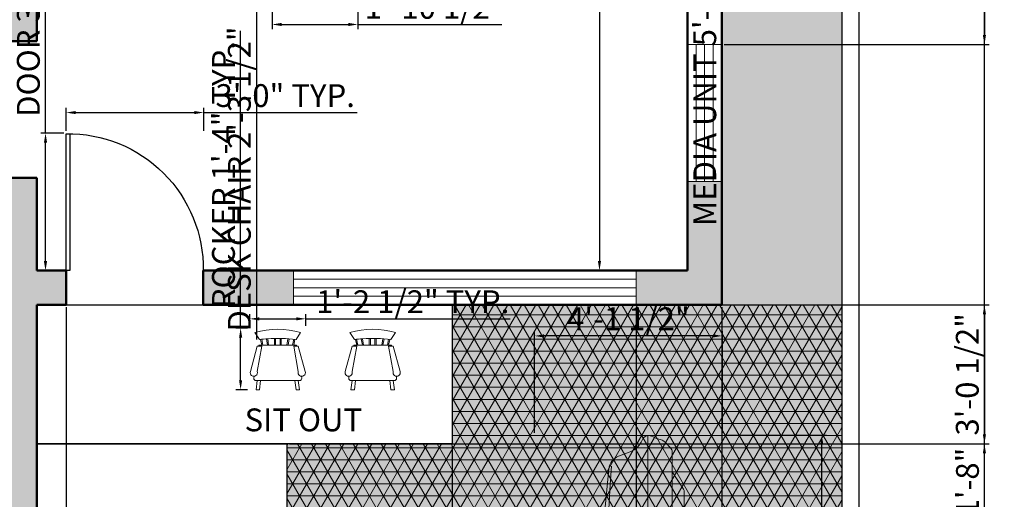
# Model space of a CAD drawing. Units: inches. Extents: x 2623 to 3157, y 1514 to 2273.
# Tile 3 of 6: x 2898 to 3157, y 1729 to 1856. Entities that reach past the tile are written whole.
import ezdxf

# ---------------------------------------------------------------- set-up
doc = ezdxf.new("R2010")
doc.units = ezdxf.units.IN
for name, color, linetype, lineweight in [('A-ANNO-DIMS', 2, 'Continuous', 18), ('A-AREA-IDEN', 7, 'Continuous', 25), ('A-DOOR', 4, 'Continuous', 25), ('A-FLOR', 7, 'Continuous', 25), ('A-FURN', 8, 'Continuous', 18), ('A-GLAZ', 4, 'Continuous', 20), ('A-WALL', 7, 'Continuous', 50), ('A-WALL-PATT', 252, 'Continuous', 13), ('C-PRKG', 8, 'Continuous', 20), ('C-PRKG-BASE-PATT', 51, 'Continuous', 13), ('C-PRKG-PATT', 252, 'Continuous', 13), ('C-PRKG-VEHL', 9, 'Continuous', 13), ('C-PROP', 7, 'Continuous', 25), ('L-PLNT-PATT', 9, 'Continuous', 13)]:
    doc.layers.add(name, color=color, linetype=linetype, lineweight=lineweight)
doc.styles.get("Standard").update_dxf_attribs({"font": 'arial.ttf'})
doc.dimstyles.new('ISO-25', dxfattribs={"dimtxt": 6, "dimasz": 2.5, "dimexe": 1.25, "dimexo": 0.625, "dimtad": 1, "dimdec": 1, "dimlunit": 3, "dimtxsty": 'Standard', "dimcen": 2.5, "dimadec": 0, "dimazin": 0, "dimtfac": 1, "dimtdec": 1, "dimtmove": 0, "dimatfit": 3, "dimfxl": 1, "dimarcsym": 0})

# ---------------------------------------------------------------- blocks, each defined once
blk = doc.blocks.new('Chair - Rocking')
for p, q in [((-8, -4.5), (-10, -1.5)), ((-4.5, -7), (-4.96674, -4.19951)), ((-4, -7), (-4.40532, -4.16272)), ((-1.5, -4.05012), (-1.5, -7)), ((-1, -7), (-1, -4.05012)), ((1, -7), (1, -4.04655)), ((1.5, -4.05012), (1.5, -7)), ((4, -7), (4.40187, -4.18694)), ((4.5, -7), (4.96761, -4.19437)), ((8, -4.5), (10, -1.5)), ((-9, -7.5), (-12, -18.49999)), ((-7, -7.5), (-9, -7.5)), ((-9, -18.49999), (-7, -7.5)), ((-8.23428, -6.99939), (-8.3093, -7.47958)), ((-8.23041, -7), (8.23915, -7)), ((-7.5, -4.5), (-7, -7)), ((-6.5, -7), (-7.02225, -4.43)), ((6.5, -7), (7, -4.4057)), ((7.5, -4.5), (7, -7)), ((7, -7.5), (9, -7.5)), ((9, -18.49999), (7, -7.5)), ((8.31071, -7.48854), (8.23449, -7.00073)), ((9, -7.5), (12, -18.49999)), ((-10.36644, -20.64523), (-10.5, -21.49999)), ((10.5, -21.49999), (10.3575, -20.58798)), ((-9, -22.49999), (-9.5, -26.49999)), ((0, -22.49999), (-9.5, -22.49999)), ((-8, -26.49999), (-7.5, -22.49999)), ((0, -22.49999), (9.5, -22.49999)), ((8, -26.49999), (7.5, -22.49999)), ((9, -22.49999), (9.5, -26.49999)), ((-9.5, -26.49999), (-8, -26.49999)), ((9.5, -26.49999), (8, -26.49999))]:
    blk.add_line(p, q)
for centre, radius, start, end in [((0, -34.08333), 34.08333, 72.93847, 107.0615), ((0, -68.25004), 64.25, 93.92211, 97.15267), ((0, -68.25004), 64.25, 82.84733, 93.92211), ((-10.5, -18.99999), 1.58114, 161.5651, 18.43495), ((-9.5, -21.49999), 1, 180, 270), ((10.5, -18.99999), 1.58114, 161.5651, 18.43495), ((9.5, -21.49999), 1, 270, 0)]:
    blk.add_arc(centre, radius, start, end)
blk = doc.blocks.new('Window - Wood Frame 36 in. Wide plan')
for p, q in [((0, 6), (0, 0)), ((36, 6), (36, 0)), ((0, 4.5), (36, 4.5)), ((0, 3), (36, 3)), ((0, 1.5), (36, 1.5))]:
    blk.add_line(p, q)
blk = doc.blocks.new('*D21')
at = {"layer": 'A-ANNO-DIMS', "color": 0, "lineweight": -2, "transparency": 16777216}
for p, q in [((3072.67, 1991.65), (3048.93, 1991.65)), ((3050.18, 1989.15), (3050.18, 1792.15)), ((3072.67, 1789.65), (3048.93, 1789.65))]:
    blk.add_line(p, q, dxfattribs=at)
at = {"layer": 'A-ANNO-DIMS', "color": 0, "transparency": 16777216}
for points in [[(3049.76, 1989.15), (3050.59, 1989.15), (3050.18, 1991.65)], [(3049.76, 1792.15), (3050.59, 1792.15), (3050.18, 1789.65)]]:
    blk.add_solid(points, dxfattribs=at)
at = {"layer": 'Defpoints', "color": 0, "transparency": 16777216}
for p in [(3073.3, 1991.65), (3050.18, 1789.65), (3073.3, 1789.65)]:
    blk.add_point(p, dxfattribs=at)
at = {"layer": 'A-ANNO-DIMS', "color": 0, "transparency": 16777216, "insert": (3046.49, 1890.65), "char_height": 6, "attachment_point": 5, "rotation": 90}
blk.add_mtext('16\'-10"', dxfattribs=at)
blk = doc.blocks.new('Car - sedan  side')
for p, q in [((-77.81, 49.34), (-126.58, 49.34)), ((-139.53, 35.99), (-129.64, 47.91)), ((-128.57, 32.64), (-121.22, 48.02)), ((-74.7, 48.02), (-121.22, 48.02)), ((-120.32, 34.67), (-115.67, 48.02)), ((-115.4, 34.67), (-111.74, 48.02)), ((-97.55, 47.3), (-111.94, 47.3)), ((-94.41, 34.67), (-97.73, 48.02)), ((-93.72, 34.67), (-97.04, 48.02)), ((-93.03, 34.67), (-96.34, 48.02)), ((-76.26, 47.3), (-96.16, 47.3)), ((-61.08, 34.66), (-76.26, 47.3)), ((-60.02, 34.65), (-76.07, 48.02)), ((-56.87, 35.13), (-75.48, 48.59)), ((-58.54, 34.93), (-74.99, 48.02)), ((-140.23, 34.67), (-163.88, 33.56)), ((-62.28, 34.67), (-140.23, 34.67)), ((-93.72, 19.62), (-93.72, 34.67)), ((-62.28, 34.67), (-60.02, 34.65)), ((-60.02, 34.65), (-58.54, 34.93)), ((-57.97, 31.61), (-60.02, 34.65)), ((-57.21, 35.38), (-58.54, 34.93)), ((-54.93, 34.4), (-8.75, 29.8)), ((-170.93, 22.32), (-166.81, 31.56)), ((-164.57, 31.6), (-165.48, 30.35)), ((-130.39, 24.63), (-128.57, 32.64)), ((-57.97, 19.62), (-57.97, 31.61)), ((-4.21, 24.18), (-5.42, 27.27)), ((-128.78, 24.63), (-144.79, 24.63)), ((-36.97, 24.38), (-34.94, 24.38)), ((-148.26, 21.7), (-171.11, 22.33)), ((-174, 19.51), (-174, 18.91)), ((-47.2, 19.62), (-125.23, 19.62)), ((-93.72, 12.14), (-93.72, 19.62)), ((-57.97, 12.14), (-57.97, 19.62)), ((0, 19.62), (-24.7, 19.62)), ((-160.12, 13.48), (-171.81, 16.16)), ((-159.22, 12.14), (-161.08, 13.7)), ((-155.01, 13.48), (-160.12, 13.48)), ((-51.4, 9.89), (-49.69, 15.14)), ((-4.23, 13.19), (-20.72, 13.19)), ((-9.5, 13.19), (-14.1, 10.2)), ((-3.22, 13.59), (-1.77, 14.97)), ((-147.03, 11.6), (-157.73, 11.6)), ((-50.67, 12.14), (-123.32, 12.14)), ((-94.21, 9.03), (-94.21, 12.14)), ((-58.39, 9.03), (-58.39, 12.14)), ((-20.36, 11.06), (-24.06, 9.44)), ((-18.83, 10.42), (-19.11, 10.76)), ((-120.62, 9.03), (-125.23, 9.03)), ((-45.76, 9.03), (-120.62, 9.03)), ((-14.68, 10.03), (-18.01, 10.03))]:
    blk.add_line(p, q)
at = {"const_width": 5.49}
for points in [[(-127.8, 11, -1), (-144.3, 11, -1)], [(-26.69, 11, -1), (-43.19, 11, -1)]]:
    blk.add_lwpolyline(points, format="xyb", close=True, dxfattribs=at)
for centre, radius in [((-136.05, 11), 11), ((-34.94, 11), 11), ((-136.05, 11), 5.51), ((-34.94, 11), 5.51)]:
    blk.add_circle(centre, radius)
for centre, radius, start, end in [((-126.58, 45.38), 3.97, 90, 140.3029), ((-77.81, 45.38), 3.97, 54.135, 90), ((-142.58, 38.53), 3.97, 272.6827, 320.3029), ((-54.54, 38.35), 3.97, 234.135, 264.3123), ((-163.72, 30.18), 3.38, 92.6827, 155.9736), ((-163.62, 30.91), 1.17, 91.491, 143.9553), ((-118.51, -1702.12), 1734.79, 86.34698, 91.49105), ((-9.15, 25.82), 4, 21.3107, 84.3123), ((-118.09, -2.78), 38.85, 136.3964, 152.9097), ((-144.79, 22.64), 1.98, 90, 136.3964), ((-128.78, 22.64), 1.98, 28.1371, 90), ((-157.14, 7.48), 34.14, 6.5135, 28.1371), ((-36.97, 11), 13.38, 90, 161.9732), ((-34.94, 11), 13.38, 13.5864, 90), ((0.9, 26.18), 5.49, 201.3107, 247.7048), ((-171.18, 19.51), 2.82, 88.4193, 180), ((-1.92, 19.3), 1.94, 325.3744, 67.7048), ((-171.18, 18.91), 2.82, 180, 257.0905), ((2.46, 16.28), 3.37, 145.3744, 172.3839), ((-3.82, 17.12), 2.96, 313.7173, 352.3839), ((-155.01, 16.1), 2.62, 270, 332.9097), ((-20.72, 14.43), 1.24, 193.5864, 270), ((-4.23, 14.65), 1.46, 270, 313.7173), ((-157.73, 13.93), 2.32, 230.1291, 270), ((-120.62, 11.65), 2.62, 186.5135, 270), ((-19.93, 10.09), 1.06, 39.301, 113.7159), ((-18.01, 11.09), 1.06, 219.301, 270), ((-52.58, 10.27), 1.24, 270, 341.9732), ((-14.68, 11.09), 1.06, 270, 303.047)]:
    blk.add_arc(centre, radius, start, end)
blk = doc.blocks.new('DOOR-SWING-36IN')
for p, q in [((36, 1), (0, 1)), ((0, 1), (0, 0)), ((36, 0), (36, 1)), ((0, 0), (36, 0))]:
    blk.add_line(p, q)
blk.add_arc((0.5, 0.5), 35.5, 359.1931, 90.8069)
blk = doc.blocks.new('*D39')
at = {"layer": 'A-ANNO-DIMS', "color": 0, "lineweight": -2, "transparency": 16777216}
for p, q in [((2904.66, 1825.78), (2904.66, 1893.28)), ((2909.45, 1825.78), (2903.41, 1825.78)), ((2904.66, 1792.15), (2904.66, 1823.28)), ((2909.45, 1789.65), (2903.41, 1789.65))]:
    blk.add_line(p, q, dxfattribs=at)
at = {"layer": 'A-ANNO-DIMS', "color": 0, "transparency": 16777216}
for points in [[(2904.24, 1823.28), (2905.08, 1823.28), (2904.66, 1825.78)], [(2904.24, 1792.15), (2905.08, 1792.15), (2904.66, 1789.65)]]:
    blk.add_solid(points, dxfattribs=at)
at = {"layer": 'Defpoints', "color": 0, "transparency": 16777216}
for p in [(2904.66, 1825.78), (2910.08, 1825.78), (2910.08, 1789.65)]:
    blk.add_point(p, dxfattribs=at)
at = {"layer": 'A-ANNO-DIMS', "color": 0, "transparency": 16777216, "insert": (2900.93, 1860.78), "char_height": 6, "attachment_point": 5, "rotation": 90}
blk.add_mtext('DOOR 3\'-0" TYP.', dxfattribs=at)
blk = doc.blocks.new('*D40')
at = {"layer": 'A-ANNO-DIMS', "color": 0, "lineweight": -2, "transparency": 16777216}
for p, q in [((2910.08, 1826.41), (2910.08, 1832.45)), ((2912.58, 1831.2), (2943.71, 1831.2)), ((2946.21, 1826.41), (2946.21, 1832.45)), ((2946.21, 1831.2), (2986.53, 1831.2))]:
    blk.add_line(p, q, dxfattribs=at)
at = {"layer": 'A-ANNO-DIMS', "color": 0, "transparency": 16777216}
for points in [[(2912.58, 1831.62), (2912.58, 1830.79), (2910.08, 1831.2)], [(2943.71, 1831.62), (2943.71, 1830.79), (2946.21, 1831.2)]]:
    blk.add_solid(points, dxfattribs=at)
at = {"layer": 'Defpoints', "color": 0, "transparency": 16777216}
for p in [(2946.21, 1831.2), (2910.08, 1825.78), (2946.21, 1825.78)]:
    blk.add_point(p, dxfattribs=at)
at = {"layer": 'A-ANNO-DIMS', "color": 0, "transparency": 16777216, "insert": (2967.62, 1834.89), "char_height": 6, "attachment_point": 5}
blk.add_mtext('3\'-0" TYP.', dxfattribs=at)
blk = doc.blocks.new('*D43')
at = {"layer": 'A-ANNO-DIMS', "color": 0, "lineweight": -2, "transparency": 16777216}
for p, q in [((2955.91, 1774.53), (2955.91, 1852.73)), ((2957.72, 1774.53), (2954.66, 1774.53)), ((2955.91, 1760.83), (2955.91, 1772.03)), ((2957.72, 1758.33), (2954.66, 1758.33))]:
    blk.add_line(p, q, dxfattribs=at)
at = {"layer": 'A-ANNO-DIMS', "color": 0, "transparency": 16777216}
for points in [[(2955.5, 1772.03), (2956.33, 1772.03), (2955.91, 1774.53)], [(2955.5, 1760.83), (2956.33, 1760.83), (2955.91, 1758.33)]]:
    blk.add_solid(points, dxfattribs=at)
at = {"layer": 'Defpoints', "color": 0, "transparency": 16777216}
for p in [(2955.91, 1774.53), (2958.34, 1774.53), (2958.34, 1758.33)]:
    blk.add_point(p, dxfattribs=at)
at = {"layer": 'A-ANNO-DIMS', "color": 0, "transparency": 16777216, "insert": (2952.18, 1814.88), "char_height": 6, "attachment_point": 5, "rotation": 90}
blk.add_mtext('ROCKER 1\'-4" TYP.', dxfattribs=at)
blk = doc.blocks.new('*D44')
at = {"layer": 'A-ANNO-DIMS', "color": 0, "lineweight": -2, "transparency": 16777216}
for p, q in [((2958.34, 1775.15), (2958.34, 1778.21)), ((2960.84, 1776.96), (2970.51, 1776.96)), ((2973.01, 1775.15), (2973.01, 1778.21)), ((2973.01, 1776.96), (3026.74, 1776.96))]:
    blk.add_line(p, q, dxfattribs=at)
at = {"layer": 'A-ANNO-DIMS', "color": 0, "transparency": 16777216}
for points in [[(2960.84, 1777.37), (2960.84, 1776.54), (2958.34, 1776.96)], [(2970.51, 1777.37), (2970.51, 1776.54), (2973.01, 1776.96)]]:
    blk.add_solid(points, dxfattribs=at)
at = {"layer": 'Defpoints', "color": 0, "transparency": 16777216}
for p in [(2973.01, 1776.96), (2958.34, 1774.53), (2973.01, 1774.53)]:
    blk.add_point(p, dxfattribs=at)
at = {"layer": 'A-ANNO-DIMS', "color": 0, "transparency": 16777216, "insert": (3001.12, 1780.68), "char_height": 6, "attachment_point": 5}
blk.add_mtext('1\'-2 1/2" TYP.', dxfattribs=at)
blk = doc.blocks.new('*D51')
at = {"layer": 'A-ANNO-DIMS', "color": 0, "lineweight": -2, "transparency": 16777216}
for p, q in [((2963.55, 1885.76), (2958.83, 1885.76)), ((2960.08, 1883.26), (2960.08, 1860.96)), ((2963.55, 1858.46), (2958.83, 1858.46)), ((2960.08, 1858.46), (2960.08, 1771.51))]:
    blk.add_line(p, q, dxfattribs=at)
at = {"layer": 'A-ANNO-DIMS', "color": 0, "transparency": 16777216}
for points in [[(2959.66, 1883.26), (2960.5, 1883.26), (2960.08, 1885.76)], [(2959.66, 1860.96), (2960.5, 1860.96), (2960.08, 1858.46)]]:
    blk.add_solid(points, dxfattribs=at)
at = {"layer": 'Defpoints', "color": 0, "transparency": 16777216}
for p in [(2964.18, 1885.76), (2960.08, 1858.46), (2964.18, 1858.46)]:
    blk.add_point(p, dxfattribs=at)
at = {"layer": 'A-ANNO-DIMS', "color": 0, "transparency": 16777216, "insert": (2956.35, 1813.73), "char_height": 6, "attachment_point": 5, "rotation": 90}
blk.add_mtext('DESK CHAIR 2\'-3 1/2"', dxfattribs=at)
blk = doc.blocks.new('*D52')
at = {"layer": 'A-ANNO-DIMS', "color": 0, "lineweight": -2, "transparency": 16777216}
for p, q in [((2964.18, 1857.83), (2964.18, 1853.11)), ((2986.71, 1857.83), (2986.71, 1853.11)), ((2966.68, 1854.36), (2984.21, 1854.36)), ((2986.71, 1854.36), (3024.49, 1854.36))]:
    blk.add_line(p, q, dxfattribs=at)
at = {"layer": 'A-ANNO-DIMS', "color": 0, "transparency": 16777216}
for points in [[(2966.68, 1854.78), (2966.68, 1853.95), (2964.18, 1854.36)], [(2984.21, 1854.78), (2984.21, 1853.95), (2986.71, 1854.36)]]:
    blk.add_solid(points, dxfattribs=at)
at = {"layer": 'Defpoints', "color": 0, "transparency": 16777216}
for p in [(2964.18, 1858.46), (2986.71, 1858.46), (2986.71, 1854.36)]:
    blk.add_point(p, dxfattribs=at)
at = {"layer": 'A-ANNO-DIMS', "color": 0, "transparency": 16777216, "insert": (3006.85, 1858.09), "char_height": 6, "attachment_point": 5}
blk.add_mtext('1\'-10 1/2"', dxfattribs=at)
blk = doc.blocks.new('*D53')
at = {"layer": 'A-ANNO-DIMS', "color": 0, "lineweight": -2, "transparency": 16777216}
for p, q in [((3073.92, 1930.37), (3083.55, 1930.37)), ((3082.3, 1927.87), (3082.3, 1872.87)), ((3073.92, 1870.37), (3083.55, 1870.37)), ((3082.3, 1870.37), (3082.3, 1800.19))]:
    blk.add_line(p, q, dxfattribs=at)
at = {"layer": 'A-ANNO-DIMS', "color": 0, "transparency": 16777216}
for points in [[(3081.88, 1927.87), (3082.71, 1927.87), (3082.3, 1930.37)], [(3081.88, 1872.87), (3082.71, 1872.87), (3082.3, 1870.37)]]:
    blk.add_solid(points, dxfattribs=at)
at = {"layer": 'Defpoints', "color": 0, "transparency": 16777216}
for p in [(3073.3, 1930.37), (3073.3, 1870.37), (3082.3, 1870.37)]:
    blk.add_point(p, dxfattribs=at)
at = {"layer": 'A-ANNO-DIMS', "color": 0, "transparency": 16777216, "insert": (3078.61, 1834.03), "char_height": 6, "attachment_point": 5, "rotation": 90}
blk.add_mtext('MEDIA UNIT 5\'-0"', dxfattribs=at)
blk = doc.blocks.new('*D57')
at = {"layer": 'A-ANNO-DIMS', "color": 0, "lineweight": -2, "transparency": 16777216}
for p, q in [((3083.08, 1746.36), (3109.82, 1746.36)), ((3108.57, 1574.74), (3108.57, 1743.86)), ((3083.08, 1572.24), (3109.82, 1572.24))]:
    blk.add_line(p, q, dxfattribs=at)
at = {"layer": 'A-ANNO-DIMS', "color": 0, "transparency": 16777216}
for points in [[(3108.16, 1743.86), (3108.99, 1743.86), (3108.57, 1746.36)], [(3108.16, 1574.74), (3108.99, 1574.74), (3108.57, 1572.24)]]:
    blk.add_solid(points, dxfattribs=at)
at = {"layer": 'Defpoints', "color": 0, "transparency": 16777216}
for p in [(3082.46, 1746.36), (3108.57, 1746.36), (3082.46, 1572.24)]:
    blk.add_point(p, dxfattribs=at)
at = {"layer": 'A-ANNO-DIMS', "color": 0, "transparency": 16777216, "insert": (3104.85, 1659.3), "char_height": 6, "attachment_point": 5, "rotation": 90}
blk.add_mtext('SEDAN 14\'-6"', dxfattribs=at)
blk = doc.blocks.new('*D58')
at = {"layer": 'A-ANNO-DIMS', "color": 0, "lineweight": -2, "transparency": 16777216}
for p, q in [((3033.11, 1746.98), (3033.11, 1773.72)), ((3079.96, 1772.47), (3035.61, 1772.47)), ((3082.46, 1746.98), (3082.46, 1773.72))]:
    blk.add_line(p, q, dxfattribs=at)
at = {"layer": 'A-ANNO-DIMS', "color": 0, "transparency": 16777216}
for points in [[(3035.61, 1772.89), (3035.61, 1772.06), (3033.11, 1772.47)], [(3079.96, 1772.89), (3079.96, 1772.06), (3082.46, 1772.47)]]:
    blk.add_solid(points, dxfattribs=at)
at = {"layer": 'Defpoints', "color": 0, "transparency": 16777216}
for p in [(3033.11, 1772.47), (3033.11, 1746.36), (3082.46, 1746.36)]:
    blk.add_point(p, dxfattribs=at)
at = {"layer": 'A-ANNO-DIMS', "color": 0, "transparency": 16777216, "insert": (3057.78, 1776.2), "char_height": 6, "attachment_point": 5}
blk.add_mtext('4\'-1 1/2"', dxfattribs=at)
blk = doc.blocks.new('*D60')
at = {"layer": 'A-ANNO-DIMS', "color": 0, "lineweight": -2, "transparency": 16777216}
for p, q in [((3118.92, 2212.65), (3152.55, 2212.65)), ((3151.3, 1555.15), (3151.3, 2210.15)), ((3118.92, 1552.65), (3152.55, 1552.65))]:
    blk.add_line(p, q, dxfattribs=at)
at = {"layer": 'A-ANNO-DIMS', "color": 0, "transparency": 16777216}
for points in [[(3150.88, 2210.15), (3151.71, 2210.15), (3151.3, 2212.65)], [(3150.88, 1555.15), (3151.71, 1555.15), (3151.3, 1552.65)]]:
    blk.add_solid(points, dxfattribs=at)
at = {"layer": 'Defpoints', "color": 0, "transparency": 16777216}
for p in [(3118.3, 2212.65), (3151.3, 2212.65), (3118.3, 1552.65)]:
    blk.add_point(p, dxfattribs=at)
at = {"layer": 'A-ANNO-DIMS', "color": 0, "transparency": 16777216, "insert": (3147.61, 1882.65), "char_height": 6, "attachment_point": 5, "rotation": 90}
blk.add_mtext('55\'-0"', dxfattribs=at)
blk = doc.blocks.new('*D66')
at = {"layer": 'A-ANNO-DIMS', "color": 0, "lineweight": -2, "transparency": 16777216}
for p, q in [((2903, 1780.65), (3152.55, 1780.65)), ((3151.3, 1615.15), (3151.3, 1778.15)), ((2903, 1612.65), (3152.55, 1612.65))]:
    blk.add_line(p, q, dxfattribs=at)
at = {"layer": 'A-ANNO-DIMS', "color": 0, "transparency": 16777216}
for points in [[(3150.88, 1778.15), (3151.71, 1778.15), (3151.3, 1780.65)], [(3150.88, 1615.15), (3151.71, 1615.15), (3151.3, 1612.65)]]:
    blk.add_solid(points, dxfattribs=at)
at = {"layer": 'Defpoints', "color": 0, "transparency": 16777216}
for p in [(2902.38, 1780.65), (3151.3, 1780.65), (2902.38, 1612.65)]:
    blk.add_point(p, dxfattribs=at)
at = {"layer": 'A-ANNO-DIMS', "color": 0, "transparency": 16777216, "insert": (3147.61, 1696.65), "char_height": 6, "attachment_point": 5, "rotation": 90}
blk.add_mtext('14\'-0"', dxfattribs=at)
blk = doc.blocks.new('*D71')
at = {"layer": 'A-ANNO-DIMS', "color": 0, "lineweight": -2, "transparency": 16777216}
for p, q in [((2902.38, 1743.46), (2902.38, 1518.4)), ((3011.52, 1743.46), (3011.52, 1518.4)), ((2904.88, 1519.65), (3009.02, 1519.65))]:
    blk.add_line(p, q, dxfattribs=at)
at = {"layer": 'A-ANNO-DIMS', "color": 0, "transparency": 16777216}
for points in [[(2904.88, 1520.06), (2904.88, 1519.23), (2902.38, 1519.65)], [(3009.02, 1520.06), (3009.02, 1519.23), (3011.52, 1519.65)]]:
    blk.add_solid(points, dxfattribs=at)
at = {"layer": 'Defpoints', "color": 0, "transparency": 16777216}
for p in [(2902.38, 1744.09), (3011.52, 1744.09), (3011.52, 1519.65)]:
    blk.add_point(p, dxfattribs=at)
at = {"layer": 'A-ANNO-DIMS', "color": 0, "transparency": 16777216, "insert": (2956.95, 1523.33), "char_height": 6, "attachment_point": 5}
blk.add_mtext('9\'-1"', dxfattribs=at)
blk = doc.blocks.new('*D72')
at = {"layer": 'A-ANNO-DIMS', "color": 0, "lineweight": -2, "transparency": 16777216}
for p, q in [((3012.14, 1780.65), (3152.55, 1780.65)), ((3151.3, 1778.15), (3151.3, 1746.59)), ((3012.14, 1744.09), (3152.55, 1744.09))]:
    blk.add_line(p, q, dxfattribs=at)
at = {"layer": 'A-ANNO-DIMS', "color": 0, "transparency": 16777216}
for points in [[(3150.88, 1778.15), (3151.71, 1778.15), (3151.3, 1780.65)], [(3150.88, 1746.59), (3151.71, 1746.59), (3151.3, 1744.09)]]:
    blk.add_solid(points, dxfattribs=at)
at = {"layer": 'Defpoints', "color": 0, "transparency": 16777216}
for p in [(3011.52, 1780.65), (3011.52, 1744.09), (3151.3, 1744.09)]:
    blk.add_point(p, dxfattribs=at)
at = {"layer": 'A-ANNO-DIMS', "color": 0, "transparency": 16777216, "insert": (3147.57, 1762.37), "char_height": 6, "attachment_point": 5, "rotation": 90}
blk.add_mtext('3\'-0 1/2"', dxfattribs=at)
blk = doc.blocks.new('*D73')
at = {"layer": 'A-ANNO-DIMS', "color": 0, "lineweight": -2, "transparency": 16777216}
for p, q in [((2968.72, 1744.09), (3152.55, 1744.09)), ((3151.3, 1726.52), (3151.3, 1741.59)), ((2968.72, 1724.02), (3152.55, 1724.02))]:
    blk.add_line(p, q, dxfattribs=at)
at = {"layer": 'A-ANNO-DIMS', "color": 0, "transparency": 16777216}
for points in [[(3150.88, 1741.59), (3151.71, 1741.59), (3151.3, 1744.09)], [(3150.88, 1726.52), (3151.71, 1726.52), (3151.3, 1724.02)]]:
    blk.add_solid(points, dxfattribs=at)
at = {"layer": 'Defpoints', "color": 0, "transparency": 16777216}
for p in [(2968.09, 1744.09), (3151.3, 1744.09), (2968.09, 1724.02)]:
    blk.add_point(p, dxfattribs=at)
at = {"layer": 'A-ANNO-DIMS', "color": 0, "transparency": 16777216, "insert": (3147.61, 1734.05), "char_height": 6, "attachment_point": 5, "rotation": 90}
blk.add_mtext('1\'-8"', dxfattribs=at)
blk = doc.blocks.new('*D83')
at = {"layer": 'A-ANNO-DIMS', "color": 0, "lineweight": -2, "transparency": 16777216}
for p, q in [((2902.38, 1780.02), (2902.38, 1518.4)), ((2910.08, 1780.02), (2910.08, 1518.4)), ((2904.88, 1519.65), (2907.58, 1519.65)), ((2910.08, 1519.65), (2943.76, 1519.65))]:
    blk.add_line(p, q, dxfattribs=at)
at = {"layer": 'A-ANNO-DIMS', "color": 0, "transparency": 16777216}
for points in [[(2904.88, 1520.06), (2904.88, 1519.23), (2902.38, 1519.65)], [(2907.58, 1520.06), (2907.58, 1519.23), (2910.08, 1519.65)]]:
    blk.add_solid(points, dxfattribs=at)
at = {"layer": 'Defpoints', "color": 0, "transparency": 16777216}
for p in [(2902.38, 1780.65), (2910.08, 1780.65), (2910.08, 1519.65)]:
    blk.add_point(p, dxfattribs=at)
at = {"layer": 'A-ANNO-DIMS', "color": 0, "transparency": 16777216, "insert": (2928.17, 1523.37), "char_height": 6, "attachment_point": 5}
blk.add_mtext('0\'-7 1/2"', dxfattribs=at)
blk = doc.blocks.new('*D84')
at = {"layer": 'A-ANNO-DIMS', "color": 0, "lineweight": -2, "transparency": 16777216}
for p, q in [((3059.78, 1780.02), (3059.78, 1518.4)), ((3082.3, 1780.02), (3082.3, 1518.4)), ((3062.28, 1519.65), (3079.8, 1519.65)), ((3082.3, 1519.65), (3120.07, 1519.65))]:
    blk.add_line(p, q, dxfattribs=at)
at = {"layer": 'A-ANNO-DIMS', "color": 0, "transparency": 16777216}
for points in [[(3062.28, 1520.06), (3062.28, 1519.23), (3059.78, 1519.65)], [(3079.8, 1520.06), (3079.8, 1519.23), (3082.3, 1519.65)]]:
    blk.add_solid(points, dxfattribs=at)
at = {"layer": 'Defpoints', "color": 0, "transparency": 16777216}
for p in [(3059.78, 1780.65), (3082.3, 1780.65), (3082.3, 1519.65)]:
    blk.add_point(p, dxfattribs=at)
at = {"layer": 'A-ANNO-DIMS', "color": 0, "transparency": 16777216, "insert": (3102.43, 1523.37), "char_height": 6, "attachment_point": 5}
blk.add_mtext('1\'-10 1/2"', dxfattribs=at)
blk = doc.blocks.new('*D95')
at = {"layer": 'A-ANNO-DIMS', "color": 0, "lineweight": -2, "transparency": 16777216}
for p, q in [((3082.92, 1938.57), (3152.55, 1938.57)), ((3151.3, 1936.07), (3151.3, 1851.59)), ((3082.92, 1849.09), (3152.55, 1849.09))]:
    blk.add_line(p, q, dxfattribs=at)
at = {"layer": 'A-ANNO-DIMS', "color": 0, "transparency": 16777216}
for points in [[(3150.88, 1936.07), (3151.71, 1936.07), (3151.3, 1938.57)], [(3150.88, 1851.59), (3151.71, 1851.59), (3151.3, 1849.09)]]:
    blk.add_solid(points, dxfattribs=at)
at = {"layer": 'Defpoints', "color": 0, "transparency": 16777216}
for p in [(3082.3, 1938.57), (3082.3, 1849.09), (3151.3, 1849.09)]:
    blk.add_point(p, dxfattribs=at)
at = {"layer": 'A-ANNO-DIMS', "color": 0, "transparency": 16777216, "insert": (3147.57, 1893.83), "char_height": 6, "attachment_point": 5, "rotation": 90}
blk.add_mtext('7\'-5 1/2"', dxfattribs=at)

msp = doc.modelspace()

# ---------------------------------------------------------------- hatches: boundary and pattern name
at = {"layer": 'A-WALL-PATT'}
h = msp.add_hatch(color=256, dxfattribs=at)
h.dxf.hatch_style = 1
h.paths.add_polyline_path([(2704.3, 1854.65), (2893.38, 1854.65), (2893.38, 1850.02), (2902.38, 1850.02), (2902.38, 1863.65), (2704.3, 1863.65), (2704.3, 1949.25), (2695.3, 1949.25), (2695.3, 1845.57), (2704.3, 1845.57)])
h.paths.add_polyline_path([(2704.3, 1809.57), (2695.3, 1809.57), (2695.3, 1750.74), (2704.3, 1750.74)])
h.paths.add_polyline_path([(2764.7, 1621.65), (2704.3, 1621.65), (2704.3, 1660.74), (2695.3, 1660.74), (2695.3, 1612.65), (2764.7, 1612.65)])
h.paths.add_polyline_path([(2704.3, 2128.1), (2695.3, 2128.1), (2695.3, 2039.25), (2704.3, 2039.25)])
h.paths.add_polyline_path([(2714, 2185.65), (2695.3, 2185.65), (2695.3, 2164.1), (2704.3, 2164.1), (2704.3, 2176.65), (2714, 2176.65)])
h.paths.add_polyline_path([(2797.66, 2185.65), (2768, 2185.65), (2768, 2176.65), (2797.66, 2176.65)])
h.paths.add_polyline_path([(2777.8, 2176.65), (2773.3, 2176.65), (2773.3, 2142.65), (2777.8, 2142.65)])
h.paths.add_polyline_path([(2963.13, 2185.65), (2887.66, 2185.65), (2887.66, 2176.65), (2963.13, 2176.65)])
h.paths.add_polyline_path([(2928.3, 2176.65), (2919.3, 2176.65), (2919.3, 2047.65), (2850.8, 2047.65), (2850.8, 2038.65), (2919.3, 2038.65), (2919.3, 2031.57), (2928.3, 2031.57), (2928.3, 2038.65)])
h.paths.add_polyline_path([(3082.3, 2185.65), (3053.13, 2185.65), (3053.13, 2176.65), (3073.3, 2176.65), (3073.3, 2169.26), (3082.3, 2169.26)])
h.paths.add_polyline_path([(3082.3, 2133.26), (3073.3, 2133.26), (3073.3, 2047.65), (2977.8, 2047.65), (2977.8, 2074.51), (2973.3, 2074.51), (2973.3, 2047.65), (2973.3, 2038.65), (2973.3, 2021.33), (2977.8, 2021.33), (2977.8, 2038.65), (3005.74, 2038.65, -0.027912), (3007.41, 2038.69, -0.0118), (3008.11, 2038.65), (3073.3, 2038.65), (3073.3, 2034.16), (3082.3, 2034.16)])
h.paths.add_polyline_path([(3082.3, 1998.16), (3073.3, 1998.16), (3073.3, 1991.65), (2977.8, 1991.65), (2977.8, 1997.33), (2973.3, 1997.33), (2973.3, 1991.65), (2928.3, 1991.65), (2928.3, 1995.57), (2919.3, 1995.57), (2919.3, 1982.65), (3073.3, 1982.65), (3073.3, 1974.57), (3082.3, 1974.57)])
h = msp.add_hatch(color=256, dxfattribs=at)
h.dxf.hatch_style = 1
h.paths.add_polyline_path([(3082.3, 1813.09), (3073.3, 1813.09), (3073.3, 1789.65), (3059.78, 1789.65), (3059.78, 1780.65), (3082.3, 1780.65)])
h.paths.add_polyline_path([(2969.78, 1789.65), (2946.08, 1789.65), (2946.08, 1780.65), (2969.78, 1780.65)])
h.paths.add_polyline_path([(2910.08, 1789.65), (2902.38, 1789.65), (2902.38, 1814.02), (2893.38, 1814.02), (2893.38, 1621.65), (2854.7, 1621.65), (2854.7, 1612.65), (2902.38, 1612.65), (2902.38, 1780.65), (2910.08, 1780.65)])
at = {"layer": 'C-PRKG-BASE-PATT'}
h = msp.add_hatch(color=256, dxfattribs=at)
h.dxf.hatch_style = 1
h.paths.add_polyline_path([(3113.8, 1780.65), (3082.3, 1780.65), (3011.52, 1780.65), (3011.52, 1744.09), (2968.09, 1744.09), (2968.09, 1724.02), (2902.38, 1724.02), (2902.38, 1557.15), (2935.08, 1557.15), (2935.08, 1552.65), (3101.15, 1552.65), (3101.15, 1557.15), (3113.8, 1557.15)])
h.paths.add_polyline_path([(3024.32, 1587.38), (2994.86, 1587.38), (2994.86, 1726.09), (3024.32, 1726.09)], flags=16)
h.paths.add_polyline_path([(3017.09, 1623.1), (3017.09, 1685.59), (2998.55, 1685.59), (2998.55, 1623.1)], flags=8)
at = {"layer": 'C-PRKG-PATT'}
h = msp.add_hatch(dxfattribs=at)
h.set_pattern_fill('NET3', color=256)
h.paths.add_polyline_path([(3113.8, 1780.65), (3082.3, 1780.65), (3011.52, 1780.65), (3011.52, 1744.09), (2968.09, 1744.09), (2968.09, 1724.02), (2902.38, 1724.02), (2902.38, 1557.15), (2935.08, 1557.15), (2935.08, 1552.65), (3101.15, 1552.65), (3101.15, 1557.15), (3113.8, 1557.15)])
h.paths.add_polyline_path([(2994.86, 1726.09), (3024.32, 1726.09), (3024.32, 1587.38), (2994.86, 1587.38)], flags=16)
h.paths.add_polyline_path([(3017.09, 1623.1), (3017.09, 1685.59), (2998.55, 1685.59), (2998.55, 1623.1)], flags=8)
at = {"layer": 'L-PLNT-PATT'}
h = msp.add_hatch(color=256, dxfattribs=at)
h.dxf.hatch_style = 1
h.set_gradient(color1=(19, 155, 72), color2=(63, 255, 0), name='CURVED')
h.paths.add_polyline_path([(2902.38, 1612.65), (2695.3, 1612.65), (2695.3, 2185.65), (3082.3, 2185.65), (3082.3, 1780.65), (3113.8, 1780.65), (3113.8, 2208.15), (2672.8, 2208.15), (2672.8, 1557.15), (2902.38, 1557.15)])
h = msp.add_hatch(color=256, dxfattribs=at)
h.dxf.hatch_style = 1
h.set_gradient(color1=(19, 155, 72), color2=(63, 255, 0), name='CYLINDER')
h.paths.add_polyline_path([(3024.32, 1726.09), (2994.86, 1726.09), (2994.86, 1587.38), (3024.32, 1587.38)], flags=17)
h.paths.add_polyline_path([(2902.38, 1612.65), (2695.3, 1612.65), (2695.3, 2185.65), (3082.3, 2185.65), (3082.3, 1780.65), (3113.8, 1780.65), (3113.8, 2208.15), (2672.8, 2208.15), (2672.8, 1557.15), (2902.38, 1557.15)])

# ---------------------------------------------------------------- linework, layer by layer
at = {"layer": 'A-FLOR'}
msp.add_line((2968.09, 1744.09), (2968.09, 1724.02), dxfattribs=at)
for points in [[(2902.38, 1780.65), (3011.52, 1780.65), (3011.52, 1744.09), (2902.38, 1744.09)], [(2902.38, 1744.09), (2968.09, 1744.09), (2968.09, 1724.02), (2902.38, 1724.02)]]:
    msp.add_lwpolyline(points, close=True, dxfattribs=at)
at = {"layer": 'A-GLAZ'}
for p, q in [((3073.3, 1849.09), (3082.3, 1849.09)), ((3073.3, 1813.09), (3082.3, 1813.09)), ((2969.78, 1789.65), (2969.78, 1780.65)), ((3059.78, 1789.65), (3059.78, 1780.65))]:
    msp.add_line(p, q, dxfattribs=at)
at = {"layer": 'A-WALL'}
for p, q in [((3082.3, 2185.65), (3082.3, 1780.65)), ((3073.3, 1991.65), (3073.3, 1789.65)), ((3073.3, 1982.65), (3073.3, 1789.65)), ((2902.38, 1850.02), (2902.38, 1863.65)), ((2893.38, 1850.02), (2902.38, 1850.02)), ((2902.38, 1814.02), (2893.38, 1814.02)), ((2902.38, 1789.65), (2902.38, 1814.02)), ((2902.38, 1789.65), (2910.08, 1789.65)), ((2910.08, 1789.65), (2910.08, 1780.65)), ((2946.08, 1780.65), (2946.08, 1789.65)), ((2946.08, 1789.65), (3073.3, 1789.65)), ((2902.38, 1612.65), (2902.38, 1780.65)), ((2902.38, 1780.65), (2910.08, 1780.65)), ((2946.08, 1780.65), (3082.3, 1780.65))]:
    msp.add_line(p, q, dxfattribs=at)
at = {"layer": 'C-PRKG'}
for p, q in [((3113.8, 1780.65), (3082.3, 1780.65)), ((3113.8, 1557.15), (3113.8, 1780.65))]:
    msp.add_line(p, q, dxfattribs=at)
at = {"layer": 'C-PROP'}
for p, q in [((3118.3, 2212.65), (3118.3, 1552.65)), ((3113.8, 2208.15), (3113.8, 1557.15))]:
    msp.add_line(p, q, dxfattribs=at)

# ---------------------------------------------------------------- block references
at = {"layer": 'A-DOOR', "extrusion": (0, 0, -1), "zscale": -1, "rotation": 89.99999999999665}
msp.add_blockref('DOOR-SWING-36IN', (-2910.08, 1789.65), dxfattribs=at)
at = {"layer": 'A-FURN', "xscale": 0.6, "yscale": 0.6}
for p in [(2965.67, 1774.23), (2990.6, 1774.23)]:
    msp.add_blockref('Chair - Rocking', p, dxfattribs=at)
at = {"layer": 'A-GLAZ', "yscale": 1.5, "rotation": 90}
msp.add_blockref('Window - Wood Frame 36 in. Wide plan', (3082.3, 1813.09), dxfattribs=at)
at = {"layer": 'A-GLAZ', "xscale": 2.5, "yscale": 1.5}
msp.add_blockref('Window - Wood Frame 36 in. Wide plan', (2969.78, 1780.65), dxfattribs=at)
at = {"layer": 'C-PRKG-VEHL', "rotation": 90}
msp.add_blockref('Car - sedan  side', (3082.46, 1746.24), dxfattribs=at)

# ---------------------------------------------------------------- texts
at = {"layer": 'A-AREA-IDEN', "insert": (2956.95, 1753.39), "char_height": 6, "attachment_point": 1}
msp.add_mtext('SIT OUT', dxfattribs=at)

# ---------------------------------------------------------------- dimensions: what is measured, and where the dimension line sits
at = {"layer": 'A-ANNO-DIMS'}
for base, p1, p2, angle, override, picture, middle in [((3151.3, 2212.65), (3118.3, 1552.65), (3118.3, 2212.65), 90, {"dimdec": 1, "dimlfac": 1, "dimrnd": 0, "dimzin": 1, "dimdsep": 46, "dimlunit": 4, "dimfrac": 2}, '*D60', (3147.61, 1882.65)), ((3050.18, 1789.65), (3073.3, 1991.65), (3073.3, 1789.65), 90, {"dimclrd": 0, "dimclre": 0, "dimclrt": 0}, '*D21', (3046.49, 1890.65)), ((3151.3, 1849.09), (3082.3, 1938.57), (3082.3, 1849.09), 90, {"dimdec": 1, "dimlfac": 1, "dimrnd": 0, "dimzin": 1, "dimdsep": 46, "dimlunit": 4, "dimfrac": 2}, '*D95', (3147.57, 1893.83)), ((3033.1105, 1772.4727), (3082.4554, 1746.3557), (3033.1105, 1746.3557), 180, {"dimdec": 1, "dimlfac": 1, "dimrnd": 0, "dimzin": 1, "dimdsep": 46, "dimlunit": 4, "dimfrac": 2}, '*D58', (3057.783, 1776.2)), ((3151.3, 1780.65), (2902.38, 1612.65), (2902.38, 1780.65), 90, {"dimdec": 1, "dimlfac": 1, "dimrnd": 0, "dimzin": 1, "dimdsep": 46, "dimlunit": 4, "dimfrac": 2}, '*D66', (3147.61, 1696.65)), ((3151.3, 1744.09), (3011.52, 1780.65), (3011.52, 1744.09), 90, {"dimdec": 1, "dimlfac": 1, "dimrnd": 0, "dimzin": 1, "dimdsep": 46, "dimlunit": 4, "dimfrac": 2}, '*D72', (3147.57, 1762.37)), ((3151.3, 1744.09), (2968.09, 1724.02), (2968.09, 1744.09), 90, {"dimdec": 1, "dimlfac": 1, "dimrnd": 0, "dimzin": 1, "dimdsep": 46, "dimlunit": 4, "dimfrac": 2}, '*D73', (3147.61, 1734.05))]:
    dim = msp.add_linear_dim(base=base, p1=p1, p2=p2, angle=angle, dimstyle='ISO-25', override=override, dxfattribs=at)
    dim.commit()
    dim.dimension.update_dxf_attribs({"geometry": picture, "text_midpoint": middle})
for base, p1, p2, angle, text, picture, middle in [((3082.3, 1870.37), (3073.3, 1930.37), (3073.3, 1870.37), 270, 'MEDIA UNIT <>', '*D53', (3078.61, 1834.03)), ((2904.66, 1825.78), (2910.08, 1789.65), (2910.08, 1825.78), 90, 'DOOR <> TYP.', '*D39', (2900.93, 1860.78)), ((2960.08, 1858.46), (2964.18, 1885.76), (2964.18, 1858.46), 270, 'DESK CHAIR <>', '*D51', (2956.35, 1813.73)), ((2955.91, 1774.53), (2958.34, 1758.33), (2958.34, 1774.53), 90, 'ROCKER <> TYP.', '*D43', (2952.18, 1814.88)), ((2946.21, 1831.2), (2910.08, 1825.78), (2946.21, 1825.78), 0, '<> TYP.', '*D40', (2967.62, 1834.89)), ((3108.57, 1746.36), (3082.46, 1572.24), (3082.46, 1746.36), 90, 'SEDAN <>', '*D57', (3104.85, 1659.3))]:
    dim = msp.add_linear_dim(base=base, p1=p1, p2=p2, angle=angle, text=text, dimstyle='ISO-25', override={"dimdec": 1, "dimlfac": 1, "dimrnd": 0, "dimzin": 1, "dimdsep": 46, "dimlunit": 4, "dimfrac": 2}, dxfattribs=at)
    dim.commit()
    dim.dimension.update_dxf_attribs({"geometry": picture, "text_midpoint": middle})
for base, p1, p2, picture, middle in [((2986.71, 1854.36), (2964.18, 1858.46), (2986.71, 1858.46), '*D52', (3006.85, 1858.09)), ((2910.08, 1519.65), (2902.38, 1780.65), (2910.08, 1780.65), '*D83', (2928.17, 1523.37)), ((3082.3, 1519.65), (3059.78, 1780.65), (3082.3, 1780.65), '*D84', (3102.43, 1523.37)), ((3011.52, 1519.65), (2902.38, 1744.09), (3011.52, 1744.09), '*D71', (2956.95, 1523.33))]:
    dim = msp.add_linear_dim(base=base, p1=p1, p2=p2, dimstyle='ISO-25', override={"dimdec": 1, "dimlfac": 1, "dimrnd": 0, "dimzin": 1, "dimdsep": 46, "dimlunit": 4, "dimfrac": 2}, dxfattribs=at)
    dim.commit()
    dim.dimension.update_dxf_attribs({"geometry": picture, "text_midpoint": middle})
dim = msp.add_linear_dim(base=(2973.01, 1776.96), p1=(2958.34, 1774.53), p2=(2973.01, 1774.53), text='<> TYP.', dimstyle='ISO-25', override={"dimdec": 1, "dimlfac": 1, "dimrnd": 0, "dimzin": 1, "dimdsep": 46, "dimlunit": 4, "dimfrac": 2}, dxfattribs=at)
dim.commit()
dim.dimension.update_dxf_attribs({"geometry": '*D44', "text_midpoint": (3001.12, 1780.68)})

doc.saveas('drawing.dxf')
